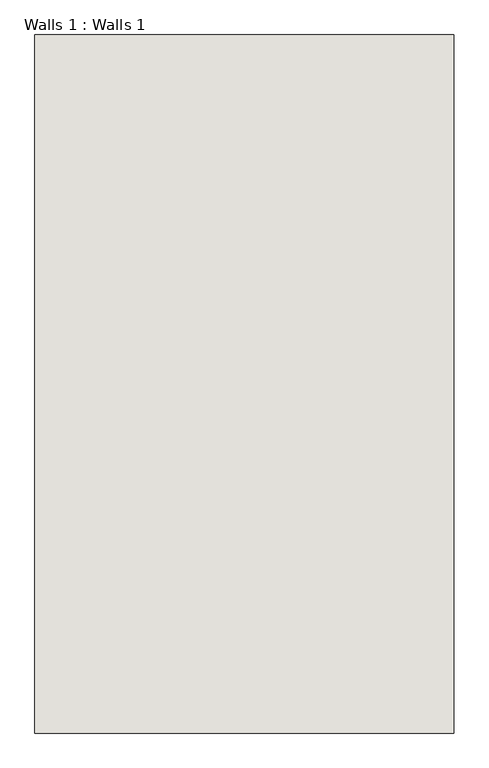
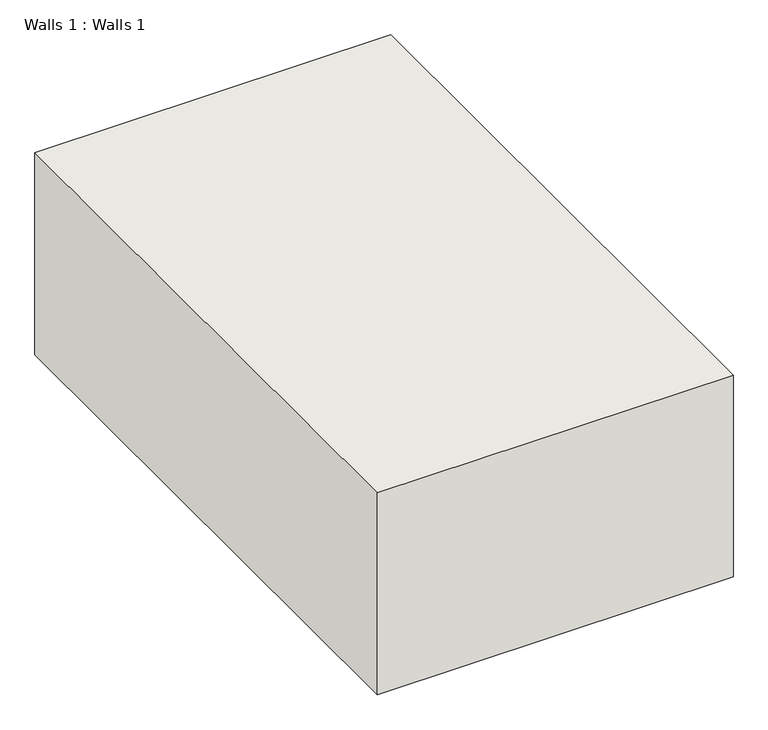
"""IFC4 building model written with IfcOpenShell, lengths in millimetres: wall geometry, Walls 1 : Walls 1."""

from ifc_helpers import new_model, si_unit, frame, origin, place, context, project, spatial, polyline, outline, extrude, source, transform, mapped, element, save


def walls_1_walls_1_4e806b56(model_context):
    return source(origin(), model_context, "Body", "SweptSolid", [
        extrude(outline(polyline([(-6134.0401579, 7262.8599287), (-6134.0401579, 12342.8599287), (-3086.0401579, 12342.8599287), (-3086.0401579, 7262.8599287), (-6134.0401579, 7262.8599287)])), frame((0.0, 0.0, -1828.8), z_axis=(0.0, 0.0, 1.0), x_axis=(1.0, 0.0, 0.0)), (0.0, 0.0, 1.0), 1828.8),
    ])


if __name__ == "__main__":
    model = new_model("IFC4")
    model_context = context("Model", 3, world=origin())
    ifc_project = project(units=[si_unit("LENGTHUNIT", "METRE", prefix="MILLI")], contexts=[model_context])
    site = spatial("IfcSite", under=ifc_project)
    building = spatial("IfcBuilding", under=site)
    placement = place(None, origin())
    walls_1_walls_1_shape = walls_1_walls_1_4e806b56(model_context)
    element("IfcWall", 1, ObjectType="Walls 1 : Walls 1", at=placement, inside=building, context=model_context, shape_type="MappedRepresentation", body=[
        mapped(walls_1_walls_1_shape, transform((0.0, 0.0, 0.0), x_axis=(1.0, 0.0, 0.0), y_axis=(0.0, 1.0, 0.0), z_axis=(0.0, 0.0, 1.0))),
    ])
    save(model, "model.ifc")

# Revit data of these elements
# Element 1 (IfcWall, "Walls 1 : Walls 1")
#   Materials on its faces: "WATER"
# Materials
#   "WATER": class "Generic", colour RGB 0 4 10, transparency 0.08, Cost = 0
